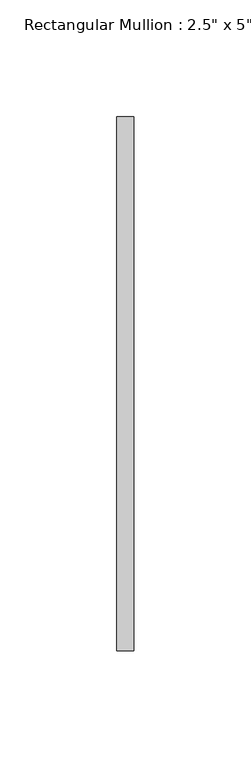
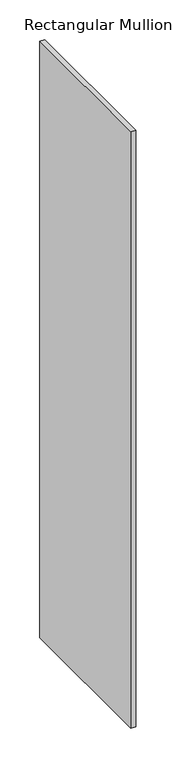
"""IFC4 building model written with IfcOpenShell, lengths in millimetres: member geometry."""

from ifc_helpers import new_model, si_unit, frame, origin, place, context, project, spatial, polyline, outline, extrude, source, transform, mapped, element, save


def member_0b5c0894(model_context):
    return source(origin(), model_context, "Body", "SweptSolid", [
        extrude(outline(polyline([(3.6195, 114.3), (3.6195, -114.3), (-3.6195, -114.3), (-3.6195, 114.3), (3.6195, 114.3)])), frame((0.0, 0.0, -914.4), z_axis=(0.0, 0.0, 1.0), x_axis=(1.0, 0.0, 0.0)), (0.0, 0.0, 1.0), 914.4),
    ])


if __name__ == "__main__":
    model = new_model("IFC4")
    model_context = context("Model", 3, world=origin())
    ifc_project = project(units=[si_unit("LENGTHUNIT", "METRE", prefix="MILLI")], contexts=[model_context])
    site = spatial("IfcSite", under=ifc_project)
    building = spatial("IfcBuilding", under=site)
    placement = place(None, origin())
    member_shape = member_0b5c0894(model_context)
    element("IfcMember", 1, ObjectType="Rectangular Mullion : 2.5\" x 5\" rectangular", at=placement, inside=building, context=model_context, shape_type="MappedRepresentation", body=[
        mapped(member_shape, transform((0.0, 0.0, 0.0), x_axis=(1.0, 0.0, 0.0), y_axis=(0.0, 1.0, 0.0), z_axis=(0.0, 0.0, 1.0))),
    ])
    save(model, "model.ifc")

# Revit data of these elements
# Type "Rectangular Mullion : 2.5\" x 5\" rectangular"
#   built-in parameter 1007304 = 0.75 (stored number, unit not read)
#   built-in parameter 1007301 = 0.011875 (stored number, unit not read)
#   built-in parameter 1007300 = 0.011875 (stored number, unit not read)
# Element 1 (IfcMember, "Rectangular Mullion : 2.5\" x 5\" rectangular")
#   Materials on its faces: "WINDOW GLASS MATERIAL"
# Materials
#   "WINDOW GLASS MATERIAL": class "Generic", colour RGB 120 120 120, transparency 0, Cost = 0
